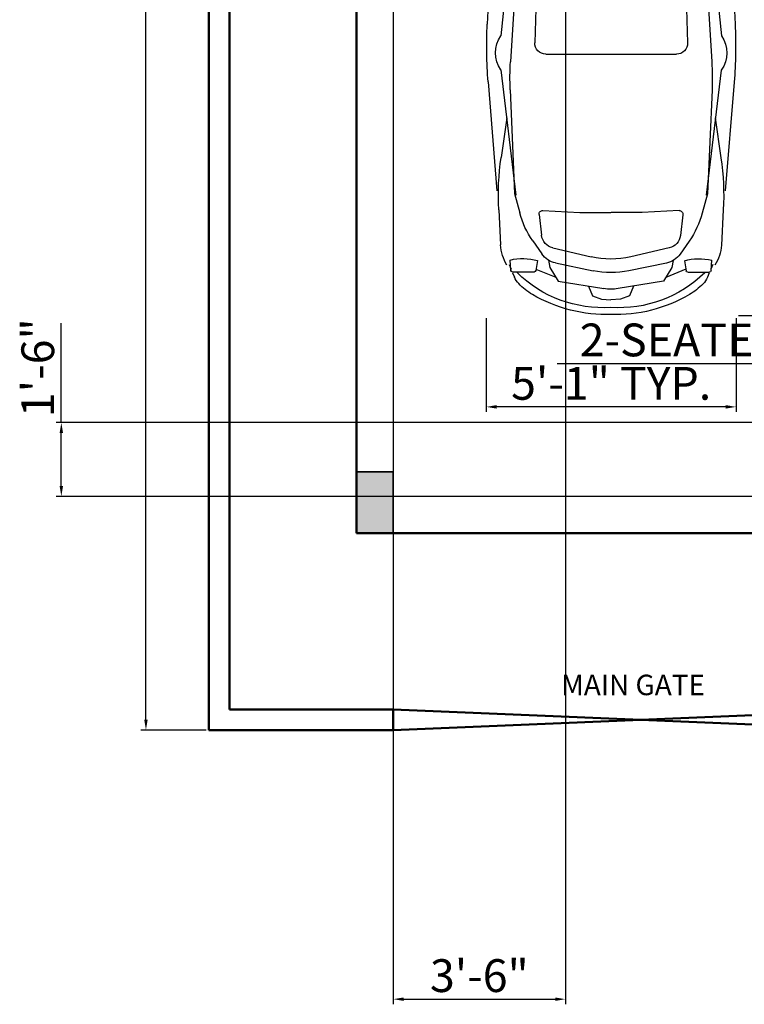
# Model space of a CAD drawing. Units: inches. Extents: x 1913 to 5309, y 1003 to 1733.
# Tile 1 of 23: x 1913 to 2090, y 1032 to 1272. Entities that reach past the tile are written whole.
import ezdxf

# ---------------------------------------------------------------- set-up
doc = ezdxf.new("R2010")
doc.units = ezdxf.units.IN
for name, color, linetype, lineweight in [('A-ANNO-DIMS', 2, 'Continuous', 18), ('A-ANNO-TEXT', 7, 'Continuous', 18), ('A-COLS', 5, 'Continuous', 35), ('A-COLS-PATT', 5, 'Continuous', 13), ('A-EQPM', 8, 'Continuous', 18), ('A-WALL', 7, 'Continuous', 50)]:
    doc.layers.add(name, color=color, linetype=linetype, lineweight=lineweight)
doc.layers.add('L9012X$0', color=2, linetype='Continuous')
doc.styles.get("Standard").update_dxf_attribs({"font": 'arial.ttf'})
doc.dimstyles.new('ISO-25', dxfattribs={"dimtxt": 8, "dimasz": 2.5, "dimexe": 1.25, "dimexo": 0.625, "dimtad": 1, "dimdec": 1, "dimlunit": 3, "dimtxsty": 'Standard', "dimcen": 2.5, "dimclrd": 256, "dimclrt": 1, "dimadec": 0, "dimazin": 0, "dimtfac": 1, "dimtdec": 1, "dimtmove": 0, "dimatfit": 3, "dimfxl": 1, "dimarcsym": 0})

# ---------------------------------------------------------------- blocks, each defined once
blk = doc.blocks.new('*D20')
at = {"layer": 'A-ANNO-DIMS', "color": 0, "lineweight": -2, "transparency": 16777216}
for p, q in [((1958.75, 1686.96), (1942.76, 1686.96)), ((1944.01, 1101.46), (1944.01, 1684.46)), ((1958.75, 1098.96), (1942.76, 1098.96))]:
    blk.add_line(p, q, dxfattribs=at)
at = {"layer": 'A-ANNO-DIMS', "color": 0, "transparency": 16777216}
for points in [[(1943.6, 1684.46), (1944.43, 1684.46), (1944.01, 1686.96)], [(1943.6, 1101.46), (1944.43, 1101.46), (1944.01, 1098.96)]]:
    blk.add_solid(points, dxfattribs=at)
at = {"layer": 'Defpoints', "color": 0, "transparency": 16777216}
for p in [(1944.01, 1686.96), (1959.37, 1686.96), (1959.37, 1098.96)]:
    blk.add_point(p, dxfattribs=at)
at = {"layer": 'A-ANNO-DIMS', "color": 0, "transparency": 16777216, "insert": (1939.3, 1392.96), "char_height": 8, "attachment_point": 5, "rotation": 90}
blk.add_mtext("49'", dxfattribs=at)
blk = doc.blocks.new('A1099DC')
at = {"color": 0, "linetype": 'ByBlock'}
for p, q in [((1279.298465, 804.448389), (2201.430588, 851.890505)), ((2602.736326, 846.078152), (3356.693814, 785.353187)), ((1475.52921, 670.226262), (2282.402739, 758.004075)), ((2519.280414, 756.817792), (3387.476361, 653.818028)), ((2851.341839, 715.213377), (3126.60716, 755.701993)), ((3488.458929, 772.663345), (3732.658862, 759.86454)), ((139.051458, 595.027331), (190.951238, 683.213377)), ((179.200345, 564.515703), (190.951238, 709.631982)), ((272.228253, 749.073842), (265.114727, 718.465169)), ((1494.603245, 682.841284), (1678.210958, 641.166865)), ((1678.210958, 641.166865), (2462.684993, 690.847736)), ((2656.476214, 692.831247), (3376.704709, 662.004075)), ((3909.27561, 688.812956), (3837.725727, 693.401722)), ((3867.794139, 700.329656), (3900.059395, 686.767505)), ((405.405047, 577.538958), (396.874865, 615.894428)), ((398.733388, 644.315148), (411.280494, 678.748261)), ((589.014326, 626.599587), (405.405047, 577.538958)), ((411.280494, 678.748261), (588.616917, 641.417897)), ((1482.852352, 674.283145), (1175.286956, 622.180789)), ((1465.665584, 620.56924), (1602.893878, 610.287296)), ((3376.704709, 662.004075), (3510.708679, 626.736433)), ((3921.162781, 527.618662), (3921.162781, 676.138994)), ((3925.383812, 676.122818), (3955.306409, 663.545364)), ((92.537504, 388.14361), (139.051458, 595.027331)), ((236.043912, 551.980927), (179.200345, 564.515703)), ((1300.814287, 466.658131), (1445.712032, 613.104998)), ((1626.354615, 583.507504), (1602.652901, 169.222264)), ((1933.148906, 509.557888), (2330.980062, 522.200075)), ((3522.252709, 492.345257), (3666.066199, 475.644444)), ((3704.596898, 536.993674), (3795.675135, 473.385795)), ((3841.786866, 503.451367), (3910.58243, 515.096797)), ((3901.001848, 514.780764), (3957.150905, 375.772812)), ((229.117398, 477.634662), (225.714299, 427.957563)), ((1860.238743, -448.635916), (1859.369151, 433.397797)), ((2409.60024, 445.938054), (2410.49349, -460.09121)), ((3493.960271, 465.734554), (3507.923021, 209.166865)), ((3839.396146, 426.841284), (3888.358202, 417.538958)), ((3888.358202, 417.538958), (3983.199613, 359.957848)), ((57.774444, 216.608726), (92.537504, 388.14361)), ((1235.045743, 136.116317), (1257.419842, 373.755108)), ((3753.293176, 397.789551), (3815.226005, 132.124765)), ((3857.610793, 379.525702), (3912.067615, 118.157673)), ((3983.199613, 359.957848), (4035.448301, 43.94997)), ((49.168662, 58.00681), (57.774444, 216.608726)), ((3507.923021, 209.166865), (3507.64153, -4.333678)), ((4019.086894, 150.376168), (4084.69605, 122.469191)), ((4084.69605, 122.469191), (4109.177079, 60.329656)), ((4109.177079, 60.329656), (4113.094043, -5.158716)), ((3508.347273, -221.154823), (3507.644805, -7.65525)), ((3983.920268, -371.008369), (4035.545755, -54.898082)), ((4109.306686, -71.132359), (4113.094514, -5.636391)), ((49.301278, -76.507426), (58.219773, -235.092064)), ((3858.370276, -390.823819), (3912.311631, -129.348921)), ((4019.394229, -161.356334), (4084.948231, -133.320044)), ((4084.948231, -133.320044), (4109.306686, -71.132359)), ((1235.330373, -152.586046), (1258.173002, -390.180259)), ((1627.520644, -599.204785), (1603.002095, -184.967086)), ((3754.088875, -409.293325), (3815.497749, -143.506937)), ((58.219773, -235.092064), (93.320996, -406.558069)), ((3494.890446, -477.749545), (3508.347273, -221.154823)), ((93.320996, -406.558069), (140.24279, -613.349673)), ((3889.19258, -428.776374), (3983.920268, -371.008369)), ((3902.027941, -525.993061), (3957.902795, -386.874665)), ((230.077082, -495.779641), (226.576036, -446.109349)), ((3840.248961, -438.175225), (3889.19258, -428.776374)), ((1301.750547, -482.997536), (1446.936772, -629.158411)), ((1934.168526, -524.650381), (2332.023837, -536.508105)), ((3523.2353, -504.304409), (3667.01558, -487.320059)), ((3705.667171, -548.593196), (3796.61981, -484.805853)), ((3842.790735, -514.780444), (3911.609128, -526.290202)), ((3922.214148, -538.79118), (3922.506998, -687.311224)), ((140.24279, -613.349673), (192.316354, -701.433212)), ((237.150178, -570.112104), (180.331436, -582.758939)), ((180.331436, -582.758939), (192.368445, -727.851766)), ((406.561378, -595.336142), (398.106841, -633.708356)), ((590.267037, -644.034637), (406.561378, -595.336142)), ((400.0214, -662.125356), (412.636377, -696.533662)), ((412.636377, -696.533662), (589.898847, -658.853701)), ((1484.19765, -690.263206), (1176.530118, -638.767405)), ((1466.905004, -636.583294), (1604.112757, -626.030785)), ((1495.965396, -698.798158), (1679.490579, -656.761786)), ((1679.490579, -656.761786), (2464.061049, -704.895745)), ((2520.786439, -770.754078), (3388.777604, -666.042617)), ((2657.855804, -706.497136), (3378.022114, -674.249887)), ((3378.022114, -674.249887), (3511.956283, -638.718087)), ((3926.727989, -687.286725), (3956.625729, -674.650294)), ((273.723073, -767.133288), (266.549207, -736.538701)), ((1476.866524, -686.22077), (2283.911563, -772.40743)), ((2852.765183, -728.494989), (3128.109803, -768.440762)), ((3910.644841, -700.0086), (3839.104145, -704.738438)), ((3869.186159, -711.60707), (3901.424611, -697.981326)), ((2604.418191, -859.849707), (3358.254477, -797.638217)), ((3489.994314, -784.688586), (3734.168535, -771.408296)), ((1280.900818, -820.829563), (2203.124693, -866.453338))]:
    blk.add_line(p, q, dxfattribs=at)
for points in [[(-0.000783, 0.794772), (5.385043, 172.701749), (63.649891, 493.818028), (92.537504, 603.957563), (144.437284, 705.166865), (428.417214, 824.236633), (585.095796, 846.190121), (961.406447, 846.190121), (1274.27399, 797.818028), (1482.852352, 709.631982)], [(83.345007, -3.206171), (111.32237, 268.957533), (164.563706, 379.583828), (279.999271, 453.709838), (456.549665, 511.628518), (901.254996, 574.918954), (1175.286956, 622.180789), (1137.52997, 385.548359), (1118.345181, 137.317882), (1109.829198, -8.358455)], [(168.178729, 359.003083), (1030.214866, 528.397865), (1077.798844, 510.531569), (1086.170082, 475.285426), (992.832238, 91.960378), (924.218938, 35.478085), (108.447994, 6.034416)], [(0.019119, -19.392451), (5.743899, -191.288474), (64.641806, -512.289243), (93.746535, -622.371603), (145.845778, -723.478374), (430.059935, -841.987962), (586.7815, -863.632471), (963.091723, -863.198028), (1275.863278, -814.209121), (1484.26735, -725.611974)], [(83.356858, -15.227176), (111.870816, -287.335185), (165.330179, -397.856284), (280.911681, -471.754535), (457.575935, -529.324983), (902.4055, -592.045995), (1176.530118, -638.767405), (1138.306616, -402.209884), (1118.632407, -154.017717), (1109.829198, -8.358455)], [(168.904615, -377.268451), (1031.273389, -545.270714), (1078.822046, -527.310627), (1087.123771, -492.048047), (993.030273, -108.907787), (924.305735, -52.560894), (108.478017, -24.418246)]]:
    blk.add_lwpolyline(points, dxfattribs=at)
for centre, radius, start, end in [((2358.037832, -2192.08357), 3048, 85.395244, 92.945173), ((2399.99649, 588.663508), 206.166238, 54.649181, 124.776949), ((3392.740754, -1053.630025), 1828.8, 86.999806, 98.367602), ((3718.678317, 475.802507), 284.405862, 57.329946, 87.182375), ((1749.553982, 373.478072), 1524, 166.916578, 176.08111), ((2578.271641, -1134.295865), 1828.8, 87.549126, 93.623712), ((4191.049821, 605.937201), 363.988953, 166.096081, 196.353514), ((3908.462781, 676.138994), 12.7, 0, 86.330429), ((446.46332, 626.922805), 50.8, 159.97873, 192.538409), ((587.047263, 633.961317), 7.62, 284.960009, 78.112462), ((1463.767788, 595.240237), 25.4, 85.715073, 135.304647), ((3355.555414, 37.211519), 609.6, 55.070043, 75.255062), ((3320.85101, 50.338397), 847.430844, 356.245089, 44.519453), ((3896.252417, 523.051998), 152.4, 46.38363, 67.20138), ((3700.933354, 318.064082), 435.542335, 30.457681, 46.38363), ((1600.996082, 584.958293), 25.4, 356.725615, 85.715073), ((1935.569151, 433.396333), 76.2, 91.82012, 179.9989), ((2333.400307, 446.03852), 76.2, 359.924458, 91.82012), ((3519.322741, 467.114813), 25.4, 83.37601, 183.115039), ((3908.462781, 527.618662), 12.7, 279.607718, 0), ((3204.184594, 25.950693), 1011.814461, 358.069446, 30.457681), ((1409.148822, 359.469565), 152.4, 135.304647, 174.62136), ((3654.346327, 374.722669), 101.6, 13.122645, 83.37601), ((3708.414764, 348.440256), 152.4, 11.769371, 55.070043), ((4645.676894, -4.872483), 3048, 176.725615, 183.38736), ((2752.335538, -6.739118), 1524, 174.62136, 185.491615), ((3221.54491, -6.276527), 609.6, 346.99033, 13.122645), ((3315.283499, -6.18411), 609.6, 348.343604, 11.769371), ((1266.577845, -8.050136), 1219.2, 176.894161, 183.218814), ((3734.73098, -5.770579), 304.8, 350.724636, 9.388339), ((3320.962449, -62.69553), 847.430844, 315.593523, 3.867886), ((3204.248172, -38.537915), 1011.814461, 329.655294, 2.043529), ((1409.873518, -375.595566), 152.4, 185.491615, 224.808328), ((3655.096735, -386.42159), 101.6, 276.736965, 346.99033), ((3709.113243, -360.032616), 152.4, 305.042932, 348.343604), ((1936.438592, -448.484202), 76.2, 180.114076, 268.292856), ((2334.293902, -460.341926), 76.2, 268.292856, 0.188517), ((3520.255588, -479.079792), 25.4, 176.997936, 276.736965), ((1750.305335, -388.625277), 1524, 184.031865, 193.196397), ((4192.255091, -616.577407), 363.988953, 163.759461, 194.016894), ((3909.514173, -538.816222), 12.7, 0.112975, 80.505257), ((1602.165021, -600.705574), 25.4, 274.397903, 3.38736), ((3355.640902, -49.500248), 609.6, 284.857913, 305.042932), ((3701.571953, -329.671253), 435.542335, 313.729345, 329.655294), ((447.716945, -644.638934), 50.8, 167.574566, 200.134245), ((588.314493, -651.400231), 7.62, 282.000513, 75.152966), ((1464.957267, -611.258083), 25.4, 224.808328, 274.397903), ((3897.294828, -534.273643), 152.4, 292.911596, 313.729345), ((2576.048678, 1120.472221), 1828.8, 266.489263, 272.563849), ((3719.627907, -487.374382), 284.405862, 272.930601, 302.78303), ((3909.807023, -687.336265), 12.7, 273.782546, 0.112975), ((2401.171182, -602.835323), 206.166238, 235.336026, 305.463794), ((3390.675263, 1041.412497), 1828.8, 261.745373, 273.113169), ((2353.729565, 2177.823616), 3048, 267.167802, 274.717731)]:
    blk.add_arc(centre, radius, start, end, dxfattribs=at)
blk = doc.blocks.new('VI')
at = {"layer": 'L9012X$0'}
blk.add_blockref('A1099DC', (0, 0), dxfattribs=at)
blk = doc.blocks.new('*D77')
at = {"layer": 'A-ANNO-DIMS', "color": 0, "lineweight": -2, "transparency": 16777216}
for p, q in [((2206.96, 1181.12), (2206.96, 1189.59)), ((2259.21, 1181.12), (2259.21, 1189.59))]:
    blk.add_line(p, q, dxfattribs=at)
at = {"layer": 'A-ANNO-DIMS', "lineweight": -2, "transparency": 16777216}
for p, q in [((2206.96, 1188.34), (2044.37, 1188.34)), ((2256.71, 1188.34), (2209.46, 1188.34))]:
    blk.add_line(p, q, dxfattribs=at)
at = {"layer": 'A-ANNO-DIMS', "transparency": 16777216}
for points in [[(2209.46, 1188.75), (2209.46, 1187.92), (2206.96, 1188.34)], [(2256.71, 1188.75), (2256.71, 1187.92), (2259.21, 1188.34)]]:
    blk.add_solid(points, dxfattribs=at)
at = {"layer": 'Defpoints', "color": 0, "transparency": 16777216}
for p in [(2206.96, 1188.34), (2206.96, 1180.5), (2259.21, 1180.5)]:
    blk.add_point(p, dxfattribs=at)
at = {"layer": 'A-ANNO-DIMS', "color": 1, "transparency": 16777216, "insert": (2124.42, 1193.1), "char_height": 8, "attachment_point": 5}
blk.add_mtext('2-SEATER SOFA 4\'-4 1/2" TYP.', dxfattribs=at)
blk = doc.blocks.new('*D85')
at = {"layer": 'A-ANNO-DIMS', "color": 0, "lineweight": -2, "transparency": 16777216}
for p, q in [((2088.63, 1348.67), (2111.54, 1348.67)), ((2088.63, 1200.09), (2111.54, 1200.09))]:
    blk.add_line(p, q, dxfattribs=at)
at = {"layer": 'A-ANNO-DIMS', "lineweight": -2, "transparency": 16777216}
blk.add_line((2110.29, 1346.17), (2110.29, 1202.59), dxfattribs=at)
at = {"layer": 'A-ANNO-DIMS', "transparency": 16777216}
for points in [[(2109.87, 1346.17), (2110.71, 1346.17), (2110.29, 1348.67)], [(2109.87, 1202.59), (2110.71, 1202.59), (2110.29, 1200.09)]]:
    blk.add_solid(points, dxfattribs=at)
at = {"layer": 'Defpoints', "color": 0, "transparency": 16777216}
for p in [(2088, 1348.67), (2088, 1200.09), (2110.29, 1200.09)]:
    blk.add_point(p, dxfattribs=at)
at = {"layer": 'A-ANNO-DIMS', "color": 1, "transparency": 16777216, "insert": (2105.53, 1274.38), "char_height": 8, "attachment_point": 5, "rotation": 90}
blk.add_mtext('CAR 12\'-4 1/2" TYP.', dxfattribs=at)
blk = doc.blocks.new('*D86')
at = {"layer": 'A-ANNO-DIMS', "color": 0, "lineweight": -2, "transparency": 16777216}
for p, q in [((2027.06, 1199.46), (2027.06, 1176.55)), ((2088, 1199.46), (2088, 1176.55))]:
    blk.add_line(p, q, dxfattribs=at)
at = {"layer": 'A-ANNO-DIMS', "lineweight": -2, "transparency": 16777216}
blk.add_line((2085.5, 1177.8), (2029.56, 1177.8), dxfattribs=at)
at = {"layer": 'A-ANNO-DIMS', "transparency": 16777216}
for points in [[(2029.56, 1178.22), (2029.56, 1177.38), (2027.06, 1177.8)], [(2085.5, 1178.22), (2085.5, 1177.38), (2088, 1177.8)]]:
    blk.add_solid(points, dxfattribs=at)
at = {"layer": 'Defpoints', "color": 0, "transparency": 16777216}
for p in [(2027.06, 1200.09), (2088, 1200.09), (2027.06, 1177.8)]:
    blk.add_point(p, dxfattribs=at)
at = {"layer": 'A-ANNO-DIMS', "color": 1, "transparency": 16777216, "insert": (2057.53, 1182.51), "char_height": 8, "attachment_point": 5}
blk.add_mtext('5\'-1" TYP.', dxfattribs=at)
blk = doc.blocks.new('*D92')
at = {"layer": 'A-ANNO-DIMS', "color": 0, "lineweight": -2, "transparency": 16777216}
for p, q in [((2004.37, 1429.34), (2004.37, 1032.04)), ((2046.37, 1429.34), (2046.37, 1032.04))]:
    blk.add_line(p, q, dxfattribs=at)
at = {"layer": 'A-ANNO-DIMS', "lineweight": -2, "transparency": 16777216}
blk.add_line((2006.87, 1033.29), (2043.87, 1033.29), dxfattribs=at)
at = {"layer": 'A-ANNO-DIMS', "transparency": 16777216}
for points in [[(2006.87, 1033.7), (2006.87, 1032.87), (2004.37, 1033.29)], [(2043.87, 1033.7), (2043.87, 1032.87), (2046.37, 1033.29)]]:
    blk.add_solid(points, dxfattribs=at)
at = {"layer": 'Defpoints', "color": 0, "transparency": 16777216}
for p in [(2004.37, 1429.96), (2046.37, 1429.96), (2046.37, 1033.29)]:
    blk.add_point(p, dxfattribs=at)
at = {"layer": 'A-ANNO-DIMS', "color": 1, "transparency": 16777216, "insert": (2025.37, 1038), "char_height": 8, "attachment_point": 5}
blk.add_mtext('3\'-6"', dxfattribs=at)
blk = doc.blocks.new('*D100')
at = {"layer": 'A-ANNO-DIMS', "lineweight": -2, "transparency": 16777216}
for p, q in [((1923.37, 1173.96), (1923.37, 1198.23)), ((1923.37, 1158.46), (1923.37, 1171.46))]:
    blk.add_line(p, q, dxfattribs=at)
at = {"layer": 'A-ANNO-DIMS', "color": 0, "lineweight": -2, "transparency": 16777216}
for p, q in [((2156.75, 1173.96), (1922.12, 1173.96)), ((2156.75, 1155.96), (1922.12, 1155.96))]:
    blk.add_line(p, q, dxfattribs=at)
at = {"layer": 'A-ANNO-DIMS', "transparency": 16777216}
for points in [[(1922.96, 1171.46), (1923.79, 1171.46), (1923.37, 1173.96)], [(1922.96, 1158.46), (1923.79, 1158.46), (1923.37, 1155.96)]]:
    blk.add_solid(points, dxfattribs=at)
at = {"layer": 'Defpoints', "color": 0, "transparency": 16777216}
for p in [(1923.37, 1173.96), (2157.37, 1173.96), (2157.37, 1155.96)]:
    blk.add_point(p, dxfattribs=at)
at = {"layer": 'A-ANNO-DIMS', "color": 1, "transparency": 16777216, "insert": (1918.66, 1187.35), "char_height": 8, "attachment_point": 5, "rotation": 90}
blk.add_mtext('1\'-6"', dxfattribs=at)

msp = doc.modelspace()

# ---------------------------------------------------------------- hatches: boundary and pattern name
at = {"layer": 'A-COLS-PATT'}
h = msp.add_hatch(color=256, dxfattribs=at)
h.dxf.hatch_style = 1
h.paths.add_polyline_path([(2004.37, 1161.96), (1995.37, 1161.96), (1995.37, 1146.96), (2004.37, 1146.96)])

# ---------------------------------------------------------------- linework, layer by layer
at = {"layer": 'A-COLS'}
msp.add_lwpolyline([(1995.37, 1146.96), (2004.37, 1146.96), (2004.37, 1161.96), (1995.37, 1161.96)], close=True, dxfattribs=at)
at = {"layer": 'A-WALL'}
for p, q in [((1959.37, 1098.96), (1959.37, 1686.96)), ((1964.37, 1103.96), (1964.37, 1681.96)), ((1995.37, 1420.96), (1995.37, 1146.96)), ((2148.37, 1146.96), (1995.37, 1146.96)), ((1964.37, 1103.96), (2004.37, 1103.96)), ((2004.37, 1103.96), (2004.37, 1098.96)), ((2004.37, 1103.96), (2124.37, 1098.96)), ((2004.37, 1098.96), (2124.37, 1103.96)), ((2004.37, 1098.96), (1959.37, 1098.96))]:
    msp.add_line(p, q, dxfattribs=at)

# ---------------------------------------------------------------- block references
at = {"layer": 'A-EQPM', "xscale": -0.0351896714874634, "yscale": 0.0351896714874634, "zscale": 0.0351896714874634, "rotation": 90}
msp.add_blockref('VI', (2057.28, 1348.67), dxfattribs=at)

# ---------------------------------------------------------------- texts
at = {"layer": 'A-ANNO-TEXT', "insert": (2045.32, 1112.46), "char_height": 5, "attachment_point": 1}
msp.add_mtext_dynamic_manual_height_columns('{MAIN GATE}', width=86.9528, gutter_width=12.5, heights=[5.17], dxfattribs=at)

# ---------------------------------------------------------------- dimensions: what is measured, and where the dimension line sits
at = {"layer": 'A-ANNO-DIMS'}
for base, p1, p2, override, picture, middle in [((1944.01, 1686.96), (1959.37, 1098.96), (1959.37, 1686.96), {"dimclrd": 0, "dimclre": 0, "dimclrt": 0}, '*D20', (1939.3, 1392.96)), ((1923.37, 1173.96), (2157.37, 1155.96), (2157.37, 1173.96), {"dimdec": 1, "dimlfac": 1, "dimrnd": 0, "dimzin": 1, "dimdsep": 46, "dimlunit": 4, "dimfrac": 2}, '*D100', (1918.66, 1187.35))]:
    dim = msp.add_linear_dim(base=base, p1=p1, p2=p2, angle=90, dimstyle='ISO-25', override=override, dxfattribs=at)
    dim.commit()
    dim.dimension.update_dxf_attribs({"geometry": picture, "text_midpoint": middle})
dim = msp.add_linear_dim(base=(2046.37, 1033.29), p1=(2004.37, 1429.96), p2=(2046.37, 1429.96), dimstyle='ISO-25', override={"dimdec": 1, "dimlfac": 1, "dimrnd": 0, "dimzin": 1, "dimdsep": 46, "dimlunit": 4, "dimfrac": 2}, dxfattribs=at)
dim.commit()
dim.dimension.update_dxf_attribs({"geometry": '*D92', "text_midpoint": (2025.37, 1038)})
for base, p1, p2, angle, text, picture, middle in [((2110.29, 1200.09), (2088, 1348.67), (2088, 1200.09), 270, 'CAR <> TYP.', '*D85', (2105.53, 1274.38)), ((2206.9567, 1188.3369), (2259.2125, 1180.4985), (2206.9567, 1180.4985), 180, '2-SEATER SOFA <> TYP.', '*D77', (2124.4156, 1193.1011)), ((2027.06, 1177.8), (2088, 1200.09), (2027.06, 1200.09), 180, '<> TYP.', '*D86', (2057.53, 1182.51))]:
    dim = msp.add_linear_dim(base=base, p1=p1, p2=p2, angle=angle, text=text, dimstyle='ISO-25', override={"dimdec": 1, "dimrnd": 0, "dimzin": 1, "dimlunit": 4, "dimfrac": 2}, dxfattribs=at)
    dim.commit()
    dim.dimension.update_dxf_attribs({"geometry": picture, "text_midpoint": middle})

doc.saveas('drawing.dxf')
